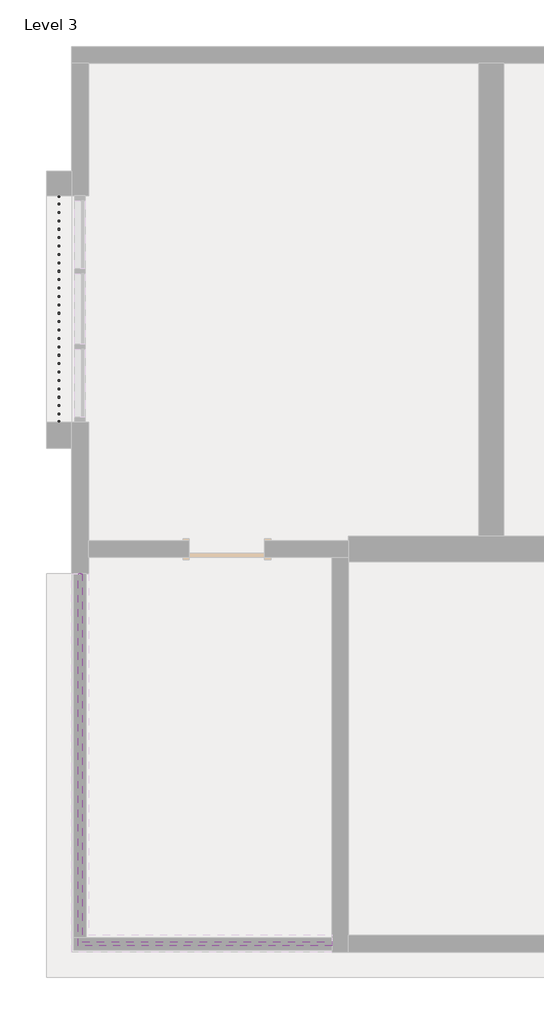
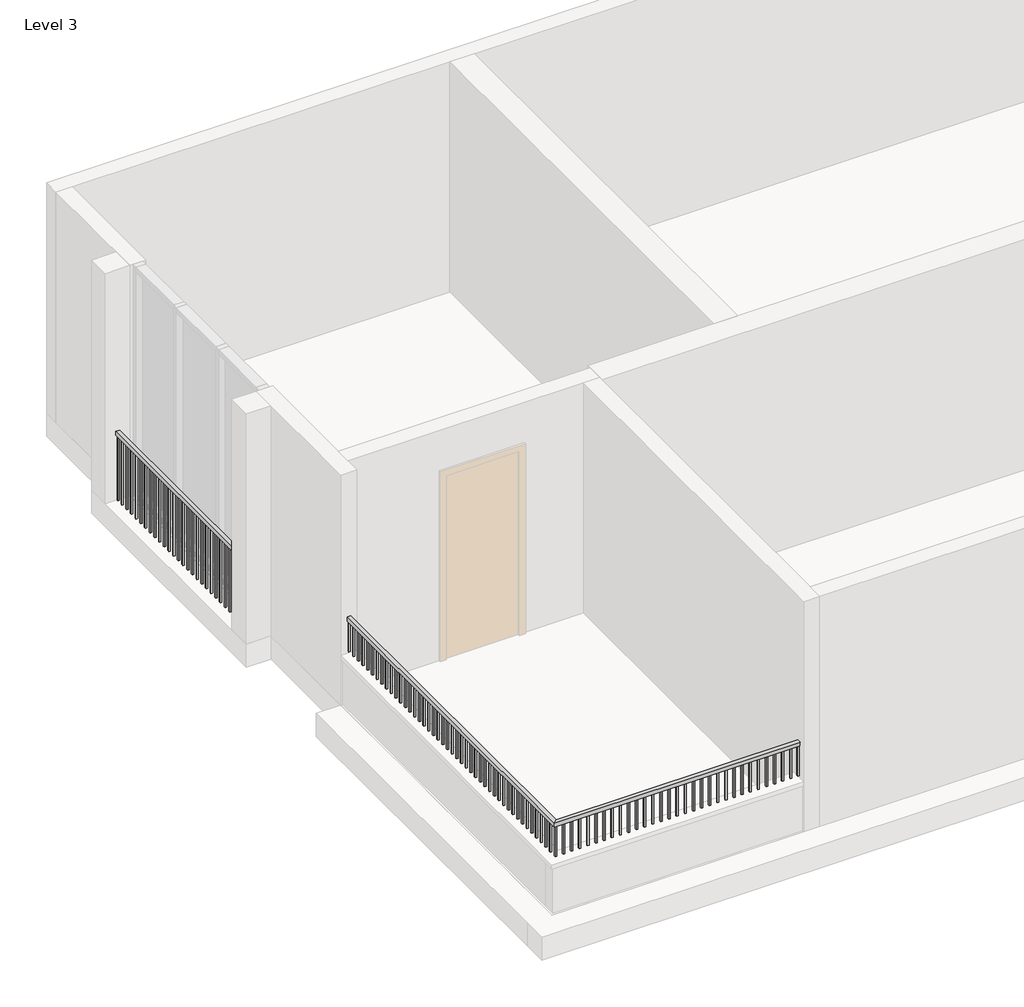
# One storey, part 2 of 2: 2 railings.
"""IFC4 building model written with IfcOpenShell, lengths in millimetres."""

from ifc_helpers import new_model, si_unit, frame, origin, place, context, project, spatial, polyline, outline, extrude, faceted_brep, element, save

model = new_model("IFC4")

# Units and contexts
model_context = context("Model", 3, world=origin())
ifc_project = project(units=[si_unit("LENGTHUNIT", "METRE", prefix="MILLI")], contexts=[model_context])

# Site, building, storey
site = spatial("IfcSite", under=ifc_project)
building = spatial("IfcBuilding", under=site)
storey = spatial("IfcBuildingStorey", under=building, Name="Level 3", Elevation=6096.0)

# Railings
placement = place(None, origin())
element("IfcRailing", 1, ObjectType="Handrail - Rectangular", at=placement, inside=storey, context=model_context, shape_type="SolidModel", body=[
    faceted_brep([(-15179.2169582, -9411.0617616, 7848.6), (-15179.2169582, -9411.0617616, 7797.8), (-15179.2169582, -9360.2617616, 7797.8), (-15179.2169582, -9360.2617616, 7848.6), (-18252.6169582, -9411.0617616, 7848.6), (-18252.6169582, -9411.0617616, 7797.8), (-18201.8169582, -9360.2617616, 7797.8), (-18201.8169582, -9360.2617616, 7848.6), (-18252.6169582, -4908.9117616, 7848.6), (-18201.8169582, -4908.9117616, 7848.6), (-18201.8169582, -4908.9117616, 7797.8), (-18252.6169582, -4908.9117616, 7797.8)], [[[0, 1, 2, 3]], [[1, 0, 4, 5]], [[2, 1, 5, 6]], [[3, 2, 6, 7]], [[0, 3, 7, 4]], [[8, 9, 10, 11]], [[5, 4, 8, 11]], [[6, 5, 11, 10]], [[7, 6, 10, 9]], [[4, 7, 9, 8]]]),
    extrude(outline(polyline([(-18217.6919582, -4924.7867616), (-18236.7419582, -4924.7867616), (-18236.7419582, -4905.7367616), (-18217.6919582, -4905.7367616), (-18217.6919582, -4924.7867616)])), frame((0.0, 0.0, 7391.4), z_axis=(0.0, 0.0, 1.0), x_axis=(1.0, 0.0, 0.0)), (0.0, 0.0, 1.0), 406.4),
    extrude(outline(polyline([(-18217.6919582, -5026.3867616), (-18236.7419582, -5026.3867616), (-18236.7419582, -5007.3367616), (-18217.6919582, -5007.3367616), (-18217.6919582, -5026.3867616)])), frame((0.0, 0.0, 7391.4), z_axis=(0.0, 0.0, 1.0), x_axis=(1.0, 0.0, 0.0)), (0.0, 0.0, 1.0), 406.4),
    extrude(outline(polyline([(-18217.6919582, -5127.9867616), (-18236.7419582, -5127.9867616), (-18236.7419582, -5108.9367616), (-18217.6919582, -5108.9367616), (-18217.6919582, -5127.9867616)])), frame((0.0, 0.0, 7391.4), z_axis=(0.0, 0.0, 1.0), x_axis=(1.0, 0.0, 0.0)), (0.0, 0.0, 1.0), 406.4),
    extrude(outline(polyline([(-18217.6919582, -5229.5867616), (-18236.7419582, -5229.5867616), (-18236.7419582, -5210.5367616), (-18217.6919582, -5210.5367616), (-18217.6919582, -5229.5867616)])), frame((0.0, 0.0, 7391.4), z_axis=(0.0, 0.0, 1.0), x_axis=(1.0, 0.0, 0.0)), (0.0, 0.0, 1.0), 406.4),
    extrude(outline(polyline([(-18217.6919582, -5331.1867616), (-18236.7419582, -5331.1867616), (-18236.7419582, -5312.1367616), (-18217.6919582, -5312.1367616), (-18217.6919582, -5331.1867616)])), frame((0.0, 0.0, 7391.4), z_axis=(0.0, 0.0, 1.0), x_axis=(1.0, 0.0, 0.0)), (0.0, 0.0, 1.0), 406.4),
    extrude(outline(polyline([(-18217.6919582, -5432.7867616), (-18236.7419582, -5432.7867616), (-18236.7419582, -5413.7367616), (-18217.6919582, -5413.7367616), (-18217.6919582, -5432.7867616)])), frame((0.0, 0.0, 7391.4), z_axis=(0.0, 0.0, 1.0), x_axis=(1.0, 0.0, 0.0)), (0.0, 0.0, 1.0), 406.4),
    extrude(outline(polyline([(-18217.6919582, -5534.3867616), (-18236.7419582, -5534.3867616), (-18236.7419582, -5515.3367616), (-18217.6919582, -5515.3367616), (-18217.6919582, -5534.3867616)])), frame((0.0, 0.0, 7391.4), z_axis=(0.0, 0.0, 1.0), x_axis=(1.0, 0.0, 0.0)), (0.0, 0.0, 1.0), 406.4),
    extrude(outline(polyline([(-18217.6919582, -5635.9867616), (-18236.7419582, -5635.9867616), (-18236.7419582, -5616.9367616), (-18217.6919582, -5616.9367616), (-18217.6919582, -5635.9867616)])), frame((0.0, 0.0, 7391.4), z_axis=(0.0, 0.0, 1.0), x_axis=(1.0, 0.0, 0.0)), (0.0, 0.0, 1.0), 406.4),
    extrude(outline(polyline([(-18217.6919582, -5737.5867616), (-18236.7419582, -5737.5867616), (-18236.7419582, -5718.5367616), (-18217.6919582, -5718.5367616), (-18217.6919582, -5737.5867616)])), frame((0.0, 0.0, 7391.4), z_axis=(0.0, 0.0, 1.0), x_axis=(1.0, 0.0, 0.0)), (0.0, 0.0, 1.0), 406.4),
    extrude(outline(polyline([(-18217.6919582, -5839.1867616), (-18236.7419582, -5839.1867616), (-18236.7419582, -5820.1367616), (-18217.6919582, -5820.1367616), (-18217.6919582, -5839.1867616)])), frame((0.0, 0.0, 7391.4), z_axis=(0.0, 0.0, 1.0), x_axis=(1.0, 0.0, 0.0)), (0.0, 0.0, 1.0), 406.4),
    extrude(outline(polyline([(-18217.6919582, -5940.7867616), (-18236.7419582, -5940.7867616), (-18236.7419582, -5921.7367616), (-18217.6919582, -5921.7367616), (-18217.6919582, -5940.7867616)])), frame((0.0, 0.0, 7391.4), z_axis=(0.0, 0.0, 1.0), x_axis=(1.0, 0.0, 0.0)), (0.0, 0.0, 1.0), 406.4),
    extrude(outline(polyline([(-18217.6919582, -6042.3867616), (-18236.7419582, -6042.3867616), (-18236.7419582, -6023.3367616), (-18217.6919582, -6023.3367616), (-18217.6919582, -6042.3867616)])), frame((0.0, 0.0, 7391.4), z_axis=(0.0, 0.0, 1.0), x_axis=(1.0, 0.0, 0.0)), (0.0, 0.0, 1.0), 406.4),
    extrude(outline(polyline([(-18217.6919582, -6143.9867616), (-18236.7419582, -6143.9867616), (-18236.7419582, -6124.9367616), (-18217.6919582, -6124.9367616), (-18217.6919582, -6143.9867616)])), frame((0.0, 0.0, 7391.4), z_axis=(0.0, 0.0, 1.0), x_axis=(1.0, 0.0, 0.0)), (0.0, 0.0, 1.0), 406.4),
    extrude(outline(polyline([(-18217.6919582, -6245.5867616), (-18236.7419582, -6245.5867616), (-18236.7419582, -6226.5367616), (-18217.6919582, -6226.5367616), (-18217.6919582, -6245.5867616)])), frame((0.0, 0.0, 7391.4), z_axis=(0.0, 0.0, 1.0), x_axis=(1.0, 0.0, 0.0)), (0.0, 0.0, 1.0), 406.4),
    extrude(outline(polyline([(-18217.6919582, -6347.1867616), (-18236.7419582, -6347.1867616), (-18236.7419582, -6328.1367616), (-18217.6919582, -6328.1367616), (-18217.6919582, -6347.1867616)])), frame((0.0, 0.0, 7391.4), z_axis=(0.0, 0.0, 1.0), x_axis=(1.0, 0.0, 0.0)), (0.0, 0.0, 1.0), 406.4),
    extrude(outline(polyline([(-18217.6919582, -6448.7867616), (-18236.7419582, -6448.7867616), (-18236.7419582, -6429.7367616), (-18217.6919582, -6429.7367616), (-18217.6919582, -6448.7867616)])), frame((0.0, 0.0, 7391.4), z_axis=(0.0, 0.0, 1.0), x_axis=(1.0, 0.0, 0.0)), (0.0, 0.0, 1.0), 406.4),
    extrude(outline(polyline([(-18217.6919582, -6550.3867616), (-18236.7419582, -6550.3867616), (-18236.7419582, -6531.3367616), (-18217.6919582, -6531.3367616), (-18217.6919582, -6550.3867616)])), frame((0.0, 0.0, 7391.4), z_axis=(0.0, 0.0, 1.0), x_axis=(1.0, 0.0, 0.0)), (0.0, 0.0, 1.0), 406.4),
    extrude(outline(polyline([(-18217.6919582, -6651.9867616), (-18236.7419582, -6651.9867616), (-18236.7419582, -6632.9367616), (-18217.6919582, -6632.9367616), (-18217.6919582, -6651.9867616)])), frame((0.0, 0.0, 7391.4), z_axis=(0.0, 0.0, 1.0), x_axis=(1.0, 0.0, 0.0)), (0.0, 0.0, 1.0), 406.4),
    extrude(outline(polyline([(-18217.6919582, -6753.5867616), (-18236.7419582, -6753.5867616), (-18236.7419582, -6734.5367616), (-18217.6919582, -6734.5367616), (-18217.6919582, -6753.5867616)])), frame((0.0, 0.0, 7391.4), z_axis=(0.0, 0.0, 1.0), x_axis=(1.0, 0.0, 0.0)), (0.0, 0.0, 1.0), 406.4),
    extrude(outline(polyline([(-18217.6919582, -6855.1867616), (-18236.7419582, -6855.1867616), (-18236.7419582, -6836.1367616), (-18217.6919582, -6836.1367616), (-18217.6919582, -6855.1867616)])), frame((0.0, 0.0, 7391.4), z_axis=(0.0, 0.0, 1.0), x_axis=(1.0, 0.0, 0.0)), (0.0, 0.0, 1.0), 406.4),
    extrude(outline(polyline([(-18217.6919582, -6956.7867616), (-18236.7419582, -6956.7867616), (-18236.7419582, -6937.7367616), (-18217.6919582, -6937.7367616), (-18217.6919582, -6956.7867616)])), frame((0.0, 0.0, 7391.4), z_axis=(0.0, 0.0, 1.0), x_axis=(1.0, 0.0, 0.0)), (0.0, 0.0, 1.0), 406.4),
    extrude(outline(polyline([(-18217.6919582, -7058.3867616), (-18236.7419582, -7058.3867616), (-18236.7419582, -7039.3367616), (-18217.6919582, -7039.3367616), (-18217.6919582, -7058.3867616)])), frame((0.0, 0.0, 7391.4), z_axis=(0.0, 0.0, 1.0), x_axis=(1.0, 0.0, 0.0)), (0.0, 0.0, 1.0), 406.4),
    extrude(outline(polyline([(-18217.6919582, -7159.9867616), (-18236.7419582, -7159.9867616), (-18236.7419582, -7140.9367616), (-18217.6919582, -7140.9367616), (-18217.6919582, -7159.9867616)])), frame((0.0, 0.0, 7391.4), z_axis=(0.0, 0.0, 1.0), x_axis=(1.0, 0.0, 0.0)), (0.0, 0.0, 1.0), 406.4),
    extrude(outline(polyline([(-18217.6919582, -7261.5867616), (-18236.7419582, -7261.5867616), (-18236.7419582, -7242.5367616), (-18217.6919582, -7242.5367616), (-18217.6919582, -7261.5867616)])), frame((0.0, 0.0, 7391.4), z_axis=(0.0, 0.0, 1.0), x_axis=(1.0, 0.0, 0.0)), (0.0, 0.0, 1.0), 406.4),
    extrude(outline(polyline([(-18217.6919582, -7363.1867616), (-18236.7419582, -7363.1867616), (-18236.7419582, -7344.1367616), (-18217.6919582, -7344.1367616), (-18217.6919582, -7363.1867616)])), frame((0.0, 0.0, 7391.4), z_axis=(0.0, 0.0, 1.0), x_axis=(1.0, 0.0, 0.0)), (0.0, 0.0, 1.0), 406.4),
    extrude(outline(polyline([(-18217.6919582, -7464.7867616), (-18236.7419582, -7464.7867616), (-18236.7419582, -7445.7367616), (-18217.6919582, -7445.7367616), (-18217.6919582, -7464.7867616)])), frame((0.0, 0.0, 7391.4), z_axis=(0.0, 0.0, 1.0), x_axis=(1.0, 0.0, 0.0)), (0.0, 0.0, 1.0), 406.4),
    extrude(outline(polyline([(-18217.6919582, -7566.3867616), (-18236.7419582, -7566.3867616), (-18236.7419582, -7547.3367616), (-18217.6919582, -7547.3367616), (-18217.6919582, -7566.3867616)])), frame((0.0, 0.0, 7391.4), z_axis=(0.0, 0.0, 1.0), x_axis=(1.0, 0.0, 0.0)), (0.0, 0.0, 1.0), 406.4),
    extrude(outline(polyline([(-18217.6919582, -7667.9867616), (-18236.7419582, -7667.9867616), (-18236.7419582, -7648.9367616), (-18217.6919582, -7648.9367616), (-18217.6919582, -7667.9867616)])), frame((0.0, 0.0, 7391.4), z_axis=(0.0, 0.0, 1.0), x_axis=(1.0, 0.0, 0.0)), (0.0, 0.0, 1.0), 406.4),
    extrude(outline(polyline([(-18217.6919582, -7769.5867616), (-18236.7419582, -7769.5867616), (-18236.7419582, -7750.5367616), (-18217.6919582, -7750.5367616), (-18217.6919582, -7769.5867616)])), frame((0.0, 0.0, 7391.4), z_axis=(0.0, 0.0, 1.0), x_axis=(1.0, 0.0, 0.0)), (0.0, 0.0, 1.0), 406.4),
    extrude(outline(polyline([(-18217.6919582, -7871.1867616), (-18236.7419582, -7871.1867616), (-18236.7419582, -7852.1367616), (-18217.6919582, -7852.1367616), (-18217.6919582, -7871.1867616)])), frame((0.0, 0.0, 7391.4), z_axis=(0.0, 0.0, 1.0), x_axis=(1.0, 0.0, 0.0)), (0.0, 0.0, 1.0), 406.4),
    extrude(outline(polyline([(-18217.6919582, -7972.7867616), (-18236.7419582, -7972.7867616), (-18236.7419582, -7953.7367616), (-18217.6919582, -7953.7367616), (-18217.6919582, -7972.7867616)])), frame((0.0, 0.0, 7391.4), z_axis=(0.0, 0.0, 1.0), x_axis=(1.0, 0.0, 0.0)), (0.0, 0.0, 1.0), 406.4),
    extrude(outline(polyline([(-18217.6919582, -8074.3867616), (-18236.7419582, -8074.3867616), (-18236.7419582, -8055.3367616), (-18217.6919582, -8055.3367616), (-18217.6919582, -8074.3867616)])), frame((0.0, 0.0, 7391.4), z_axis=(0.0, 0.0, 1.0), x_axis=(1.0, 0.0, 0.0)), (0.0, 0.0, 1.0), 406.4),
    extrude(outline(polyline([(-18217.6919582, -8175.9867616), (-18236.7419582, -8175.9867616), (-18236.7419582, -8156.9367616), (-18217.6919582, -8156.9367616), (-18217.6919582, -8175.9867616)])), frame((0.0, 0.0, 7391.4), z_axis=(0.0, 0.0, 1.0), x_axis=(1.0, 0.0, 0.0)), (0.0, 0.0, 1.0), 406.4),
    extrude(outline(polyline([(-18217.6919582, -8277.5867616), (-18236.7419582, -8277.5867616), (-18236.7419582, -8258.5367616), (-18217.6919582, -8258.5367616), (-18217.6919582, -8277.5867616)])), frame((0.0, 0.0, 7391.4), z_axis=(0.0, 0.0, 1.0), x_axis=(1.0, 0.0, 0.0)), (0.0, 0.0, 1.0), 406.4),
    extrude(outline(polyline([(-18217.6919582, -8379.1867616), (-18236.7419582, -8379.1867616), (-18236.7419582, -8360.1367616), (-18217.6919582, -8360.1367616), (-18217.6919582, -8379.1867616)])), frame((0.0, 0.0, 7391.4), z_axis=(0.0, 0.0, 1.0), x_axis=(1.0, 0.0, 0.0)), (0.0, 0.0, 1.0), 406.4),
    extrude(outline(polyline([(-18217.6919582, -8480.7867616), (-18236.7419582, -8480.7867616), (-18236.7419582, -8461.7367616), (-18217.6919582, -8461.7367616), (-18217.6919582, -8480.7867616)])), frame((0.0, 0.0, 7391.4), z_axis=(0.0, 0.0, 1.0), x_axis=(1.0, 0.0, 0.0)), (0.0, 0.0, 1.0), 406.4),
    extrude(outline(polyline([(-18217.6919582, -8582.3867616), (-18236.7419582, -8582.3867616), (-18236.7419582, -8563.3367616), (-18217.6919582, -8563.3367616), (-18217.6919582, -8582.3867616)])), frame((0.0, 0.0, 7391.4), z_axis=(0.0, 0.0, 1.0), x_axis=(1.0, 0.0, 0.0)), (0.0, 0.0, 1.0), 406.4),
    extrude(outline(polyline([(-18217.6919582, -8683.9867616), (-18236.7419582, -8683.9867616), (-18236.7419582, -8664.9367616), (-18217.6919582, -8664.9367616), (-18217.6919582, -8683.9867616)])), frame((0.0, 0.0, 7391.4), z_axis=(0.0, 0.0, 1.0), x_axis=(1.0, 0.0, 0.0)), (0.0, 0.0, 1.0), 406.4),
    extrude(outline(polyline([(-18217.6919582, -8785.5867616), (-18236.7419582, -8785.5867616), (-18236.7419582, -8766.5367616), (-18217.6919582, -8766.5367616), (-18217.6919582, -8785.5867616)])), frame((0.0, 0.0, 7391.4), z_axis=(0.0, 0.0, 1.0), x_axis=(1.0, 0.0, 0.0)), (0.0, 0.0, 1.0), 406.4),
    extrude(outline(polyline([(-18217.6919582, -8887.1867616), (-18236.7419582, -8887.1867616), (-18236.7419582, -8868.1367616), (-18217.6919582, -8868.1367616), (-18217.6919582, -8887.1867616)])), frame((0.0, 0.0, 7391.4), z_axis=(0.0, 0.0, 1.0), x_axis=(1.0, 0.0, 0.0)), (0.0, 0.0, 1.0), 406.4),
    extrude(outline(polyline([(-18217.6919582, -8988.7867616), (-18236.7419582, -8988.7867616), (-18236.7419582, -8969.7367616), (-18217.6919582, -8969.7367616), (-18217.6919582, -8988.7867616)])), frame((0.0, 0.0, 7391.4), z_axis=(0.0, 0.0, 1.0), x_axis=(1.0, 0.0, 0.0)), (0.0, 0.0, 1.0), 406.4),
    extrude(outline(polyline([(-18217.6919582, -9090.3867616), (-18236.7419582, -9090.3867616), (-18236.7419582, -9071.3367616), (-18217.6919582, -9071.3367616), (-18217.6919582, -9090.3867616)])), frame((0.0, 0.0, 7391.4), z_axis=(0.0, 0.0, 1.0), x_axis=(1.0, 0.0, 0.0)), (0.0, 0.0, 1.0), 406.4),
    extrude(outline(polyline([(-18217.6919582, -9191.9867616), (-18236.7419582, -9191.9867616), (-18236.7419582, -9172.9367616), (-18217.6919582, -9172.9367616), (-18217.6919582, -9191.9867616)])), frame((0.0, 0.0, 7391.4), z_axis=(0.0, 0.0, 1.0), x_axis=(1.0, 0.0, 0.0)), (0.0, 0.0, 1.0), 406.4),
    extrude(outline(polyline([(-18217.6919582, -9293.5867616), (-18236.7419582, -9293.5867616), (-18236.7419582, -9274.5367616), (-18217.6919582, -9274.5367616), (-18217.6919582, -9293.5867616)])), frame((0.0, 0.0, 7391.4), z_axis=(0.0, 0.0, 1.0), x_axis=(1.0, 0.0, 0.0)), (0.0, 0.0, 1.0), 406.4),
    extrude(outline(polyline([(-18116.0919582, -9376.1367616), (-18116.0919582, -9395.1867616), (-18135.1419582, -9395.1867616), (-18135.1419582, -9376.1367616), (-18116.0919582, -9376.1367616)])), frame((0.0, 0.0, 7391.4), z_axis=(0.0, 0.0, 1.0), x_axis=(1.0, 0.0, 0.0)), (0.0, 0.0, 1.0), 406.4),
    extrude(outline(polyline([(-18014.4919582, -9376.1367616), (-18014.4919582, -9395.1867616), (-18033.5419582, -9395.1867616), (-18033.5419582, -9376.1367616), (-18014.4919582, -9376.1367616)])), frame((0.0, 0.0, 7391.4), z_axis=(0.0, 0.0, 1.0), x_axis=(1.0, 0.0, 0.0)), (0.0, 0.0, 1.0), 406.4),
    extrude(outline(polyline([(-17912.8919582, -9376.1367616), (-17912.8919582, -9395.1867616), (-17931.9419582, -9395.1867616), (-17931.9419582, -9376.1367616), (-17912.8919582, -9376.1367616)])), frame((0.0, 0.0, 7391.4), z_axis=(0.0, 0.0, 1.0), x_axis=(1.0, 0.0, 0.0)), (0.0, 0.0, 1.0), 406.4),
    extrude(outline(polyline([(-17811.2919582, -9376.1367616), (-17811.2919582, -9395.1867616), (-17830.3419582, -9395.1867616), (-17830.3419582, -9376.1367616), (-17811.2919582, -9376.1367616)])), frame((0.0, 0.0, 7391.4), z_axis=(0.0, 0.0, 1.0), x_axis=(1.0, 0.0, 0.0)), (0.0, 0.0, 1.0), 406.4),
    extrude(outline(polyline([(-17709.6919582, -9376.1367616), (-17709.6919582, -9395.1867616), (-17728.7419582, -9395.1867616), (-17728.7419582, -9376.1367616), (-17709.6919582, -9376.1367616)])), frame((0.0, 0.0, 7391.4), z_axis=(0.0, 0.0, 1.0), x_axis=(1.0, 0.0, 0.0)), (0.0, 0.0, 1.0), 406.4),
    extrude(outline(polyline([(-17608.0919582, -9376.1367616), (-17608.0919582, -9395.1867616), (-17627.1419582, -9395.1867616), (-17627.1419582, -9376.1367616), (-17608.0919582, -9376.1367616)])), frame((0.0, 0.0, 7391.4), z_axis=(0.0, 0.0, 1.0), x_axis=(1.0, 0.0, 0.0)), (0.0, 0.0, 1.0), 406.4),
    extrude(outline(polyline([(-17506.4919582, -9376.1367616), (-17506.4919582, -9395.1867616), (-17525.5419582, -9395.1867616), (-17525.5419582, -9376.1367616), (-17506.4919582, -9376.1367616)])), frame((0.0, 0.0, 7391.4), z_axis=(0.0, 0.0, 1.0), x_axis=(1.0, 0.0, 0.0)), (0.0, 0.0, 1.0), 406.4),
    extrude(outline(polyline([(-17404.8919582, -9376.1367616), (-17404.8919582, -9395.1867616), (-17423.9419582, -9395.1867616), (-17423.9419582, -9376.1367616), (-17404.8919582, -9376.1367616)])), frame((0.0, 0.0, 7391.4), z_axis=(0.0, 0.0, 1.0), x_axis=(1.0, 0.0, 0.0)), (0.0, 0.0, 1.0), 406.4),
    extrude(outline(polyline([(-17303.2919582, -9376.1367616), (-17303.2919582, -9395.1867616), (-17322.3419582, -9395.1867616), (-17322.3419582, -9376.1367616), (-17303.2919582, -9376.1367616)])), frame((0.0, 0.0, 7391.4), z_axis=(0.0, 0.0, 1.0), x_axis=(1.0, 0.0, 0.0)), (0.0, 0.0, 1.0), 406.4),
    extrude(outline(polyline([(-17201.6919582, -9376.1367616), (-17201.6919582, -9395.1867616), (-17220.7419582, -9395.1867616), (-17220.7419582, -9376.1367616), (-17201.6919582, -9376.1367616)])), frame((0.0, 0.0, 7391.4), z_axis=(0.0, 0.0, 1.0), x_axis=(1.0, 0.0, 0.0)), (0.0, 0.0, 1.0), 406.4),
    extrude(outline(polyline([(-17100.0919582, -9376.1367616), (-17100.0919582, -9395.1867616), (-17119.1419582, -9395.1867616), (-17119.1419582, -9376.1367616), (-17100.0919582, -9376.1367616)])), frame((0.0, 0.0, 7391.4), z_axis=(0.0, 0.0, 1.0), x_axis=(1.0, 0.0, 0.0)), (0.0, 0.0, 1.0), 406.4),
    extrude(outline(polyline([(-16998.4919582, -9376.1367616), (-16998.4919582, -9395.1867616), (-17017.5419582, -9395.1867616), (-17017.5419582, -9376.1367616), (-16998.4919582, -9376.1367616)])), frame((0.0, 0.0, 7391.4), z_axis=(0.0, 0.0, 1.0), x_axis=(1.0, 0.0, 0.0)), (0.0, 0.0, 1.0), 406.4),
    extrude(outline(polyline([(-16896.8919582, -9376.1367616), (-16896.8919582, -9395.1867616), (-16915.9419582, -9395.1867616), (-16915.9419582, -9376.1367616), (-16896.8919582, -9376.1367616)])), frame((0.0, 0.0, 7391.4), z_axis=(0.0, 0.0, 1.0), x_axis=(1.0, 0.0, 0.0)), (0.0, 0.0, 1.0), 406.4),
    extrude(outline(polyline([(-16795.2919582, -9376.1367616), (-16795.2919582, -9395.1867616), (-16814.3419582, -9395.1867616), (-16814.3419582, -9376.1367616), (-16795.2919582, -9376.1367616)])), frame((0.0, 0.0, 7391.4), z_axis=(0.0, 0.0, 1.0), x_axis=(1.0, 0.0, 0.0)), (0.0, 0.0, 1.0), 406.4),
    extrude(outline(polyline([(-16693.6919582, -9376.1367616), (-16693.6919582, -9395.1867616), (-16712.7419582, -9395.1867616), (-16712.7419582, -9376.1367616), (-16693.6919582, -9376.1367616)])), frame((0.0, 0.0, 7391.4), z_axis=(0.0, 0.0, 1.0), x_axis=(1.0, 0.0, 0.0)), (0.0, 0.0, 1.0), 406.4),
    extrude(outline(polyline([(-16592.0919582, -9376.1367616), (-16592.0919582, -9395.1867616), (-16611.1419582, -9395.1867616), (-16611.1419582, -9376.1367616), (-16592.0919582, -9376.1367616)])), frame((0.0, 0.0, 7391.4), z_axis=(0.0, 0.0, 1.0), x_axis=(1.0, 0.0, 0.0)), (0.0, 0.0, 1.0), 406.4),
    extrude(outline(polyline([(-16490.4919582, -9376.1367616), (-16490.4919582, -9395.1867616), (-16509.5419582, -9395.1867616), (-16509.5419582, -9376.1367616), (-16490.4919582, -9376.1367616)])), frame((0.0, 0.0, 7391.4), z_axis=(0.0, 0.0, 1.0), x_axis=(1.0, 0.0, 0.0)), (0.0, 0.0, 1.0), 406.4),
    extrude(outline(polyline([(-16388.8919582, -9376.1367616), (-16388.8919582, -9395.1867616), (-16407.9419582, -9395.1867616), (-16407.9419582, -9376.1367616), (-16388.8919582, -9376.1367616)])), frame((0.0, 0.0, 7391.4), z_axis=(0.0, 0.0, 1.0), x_axis=(1.0, 0.0, 0.0)), (0.0, 0.0, 1.0), 406.4),
    extrude(outline(polyline([(-16287.2919582, -9376.1367616), (-16287.2919582, -9395.1867616), (-16306.3419582, -9395.1867616), (-16306.3419582, -9376.1367616), (-16287.2919582, -9376.1367616)])), frame((0.0, 0.0, 7391.4), z_axis=(0.0, 0.0, 1.0), x_axis=(1.0, 0.0, 0.0)), (0.0, 0.0, 1.0), 406.4),
    extrude(outline(polyline([(-16185.6919582, -9376.1367616), (-16185.6919582, -9395.1867616), (-16204.7419582, -9395.1867616), (-16204.7419582, -9376.1367616), (-16185.6919582, -9376.1367616)])), frame((0.0, 0.0, 7391.4), z_axis=(0.0, 0.0, 1.0), x_axis=(1.0, 0.0, 0.0)), (0.0, 0.0, 1.0), 406.4),
    extrude(outline(polyline([(-16084.0919582, -9376.1367616), (-16084.0919582, -9395.1867616), (-16103.1419582, -9395.1867616), (-16103.1419582, -9376.1367616), (-16084.0919582, -9376.1367616)])), frame((0.0, 0.0, 7391.4), z_axis=(0.0, 0.0, 1.0), x_axis=(1.0, 0.0, 0.0)), (0.0, 0.0, 1.0), 406.4),
    extrude(outline(polyline([(-15982.4919582, -9376.1367616), (-15982.4919582, -9395.1867616), (-16001.5419582, -9395.1867616), (-16001.5419582, -9376.1367616), (-15982.4919582, -9376.1367616)])), frame((0.0, 0.0, 7391.4), z_axis=(0.0, 0.0, 1.0), x_axis=(1.0, 0.0, 0.0)), (0.0, 0.0, 1.0), 406.4),
    extrude(outline(polyline([(-15880.8919582, -9376.1367616), (-15880.8919582, -9395.1867616), (-15899.9419582, -9395.1867616), (-15899.9419582, -9376.1367616), (-15880.8919582, -9376.1367616)])), frame((0.0, 0.0, 7391.4), z_axis=(0.0, 0.0, 1.0), x_axis=(1.0, 0.0, 0.0)), (0.0, 0.0, 1.0), 406.4),
    extrude(outline(polyline([(-15779.2919582, -9376.1367616), (-15779.2919582, -9395.1867616), (-15798.3419582, -9395.1867616), (-15798.3419582, -9376.1367616), (-15779.2919582, -9376.1367616)])), frame((0.0, 0.0, 7391.4), z_axis=(0.0, 0.0, 1.0), x_axis=(1.0, 0.0, 0.0)), (0.0, 0.0, 1.0), 406.4),
    extrude(outline(polyline([(-15677.6919582, -9376.1367616), (-15677.6919582, -9395.1867616), (-15696.7419582, -9395.1867616), (-15696.7419582, -9376.1367616), (-15677.6919582, -9376.1367616)])), frame((0.0, 0.0, 7391.4), z_axis=(0.0, 0.0, 1.0), x_axis=(1.0, 0.0, 0.0)), (0.0, 0.0, 1.0), 406.4),
    extrude(outline(polyline([(-15576.0919582, -9376.1367616), (-15576.0919582, -9395.1867616), (-15595.1419582, -9395.1867616), (-15595.1419582, -9376.1367616), (-15576.0919582, -9376.1367616)])), frame((0.0, 0.0, 7391.4), z_axis=(0.0, 0.0, 1.0), x_axis=(1.0, 0.0, 0.0)), (0.0, 0.0, 1.0), 406.4),
    extrude(outline(polyline([(-15474.4919582, -9376.1367616), (-15474.4919582, -9395.1867616), (-15493.5419582, -9395.1867616), (-15493.5419582, -9376.1367616), (-15474.4919582, -9376.1367616)])), frame((0.0, 0.0, 7391.4), z_axis=(0.0, 0.0, 1.0), x_axis=(1.0, 0.0, 0.0)), (0.0, 0.0, 1.0), 406.4),
    extrude(outline(polyline([(-15372.8919582, -9376.1367616), (-15372.8919582, -9395.1867616), (-15391.9419582, -9395.1867616), (-15391.9419582, -9376.1367616), (-15372.8919582, -9376.1367616)])), frame((0.0, 0.0, 7391.4), z_axis=(0.0, 0.0, 1.0), x_axis=(1.0, 0.0, 0.0)), (0.0, 0.0, 1.0), 406.4),
    extrude(outline(polyline([(-15271.2919582, -9376.1367616), (-15271.2919582, -9395.1867616), (-15290.3419582, -9395.1867616), (-15290.3419582, -9376.1367616), (-15271.2919582, -9376.1367616)])), frame((0.0, 0.0, 7391.4), z_axis=(0.0, 0.0, 1.0), x_axis=(1.0, 0.0, 0.0)), (0.0, 0.0, 1.0), 406.4),
    extrude(outline(polyline([(-18217.6919582, -9376.1367616), (-18217.6919582, -9395.1867616), (-18236.7419582, -9395.1867616), (-18236.7419582, -9376.1367616), (-18217.6919582, -9376.1367616)])), frame((0.0, 0.0, 7391.4), z_axis=(0.0, 0.0, 1.0), x_axis=(1.0, 0.0, 0.0)), (0.0, 0.0, 1.0), 406.4),
    extrude(outline(polyline([(-18217.6919582, -4927.9617616), (-18236.7419582, -4927.9617616), (-18236.7419582, -4908.9117616), (-18217.6919582, -4908.9117616), (-18217.6919582, -4927.9617616)])), frame((0.0, 0.0, 7391.4), z_axis=(0.0, 0.0, 1.0), x_axis=(1.0, 0.0, 0.0)), (0.0, 0.0, 1.0), 406.4),
    extrude(outline(polyline([(-15179.2169582, -9376.1367616), (-15179.2169582, -9395.1867616), (-15198.2669582, -9395.1867616), (-15198.2669582, -9376.1367616), (-15179.2169582, -9376.1367616)])), frame((0.0, 0.0, 7391.4), z_axis=(0.0, 0.0, 1.0), x_axis=(1.0, 0.0, 0.0)), (0.0, 0.0, 1.0), 406.4),
])
element("IfcRailing", 2, ObjectType="Handrail - Rectangular 2", at=placement, inside=storey, context=model_context, shape_type="SweptSolid", body=[
    extrude(outline(polyline([(-18506.6169582, -336.9117616), (-18455.8169582, -336.9117616), (-18455.8169582, -3080.1117616), (-18506.6169582, -3080.1117616), (-18506.6169582, -336.9117616)])), frame((0.0, 0.0, 7569.2), z_axis=(0.0, 0.0, 1.0), x_axis=(1.0, 0.0, 0.0)), (0.0, 0.0, 1.0), 50.8),
    extrude(outline(polyline([(-18490.7419582, -2968.9867616), (-18471.6919582, -2968.9867616), (-18471.6919582, -2988.0367616), (-18490.7419582, -2988.0367616), (-18490.7419582, -2968.9867616)])), frame((0.0, 0.0, 6705.6), z_axis=(0.0, 0.0, 1.0), x_axis=(1.0, 0.0, 0.0)), (0.0, 0.0, 1.0), 863.6),
    extrude(outline(polyline([(-18490.7419582, -2867.3867616), (-18471.6919582, -2867.3867616), (-18471.6919582, -2886.4367616), (-18490.7419582, -2886.4367616), (-18490.7419582, -2867.3867616)])), frame((0.0, 0.0, 6705.6), z_axis=(0.0, 0.0, 1.0), x_axis=(1.0, 0.0, 0.0)), (0.0, 0.0, 1.0), 863.6),
    extrude(outline(polyline([(-18490.7419582, -2765.7867616), (-18471.6919582, -2765.7867616), (-18471.6919582, -2784.8367616), (-18490.7419582, -2784.8367616), (-18490.7419582, -2765.7867616)])), frame((0.0, 0.0, 6705.6), z_axis=(0.0, 0.0, 1.0), x_axis=(1.0, 0.0, 0.0)), (0.0, 0.0, 1.0), 863.6),
    extrude(outline(polyline([(-18490.7419582, -2664.1867616), (-18471.6919582, -2664.1867616), (-18471.6919582, -2683.2367616), (-18490.7419582, -2683.2367616), (-18490.7419582, -2664.1867616)])), frame((0.0, 0.0, 6705.6), z_axis=(0.0, 0.0, 1.0), x_axis=(1.0, 0.0, 0.0)), (0.0, 0.0, 1.0), 863.6),
    extrude(outline(polyline([(-18490.7419582, -2562.5867616), (-18471.6919582, -2562.5867616), (-18471.6919582, -2581.6367616), (-18490.7419582, -2581.6367616), (-18490.7419582, -2562.5867616)])), frame((0.0, 0.0, 6705.6), z_axis=(0.0, 0.0, 1.0), x_axis=(1.0, 0.0, 0.0)), (0.0, 0.0, 1.0), 863.6),
    extrude(outline(polyline([(-18490.7419582, -2460.9867616), (-18471.6919582, -2460.9867616), (-18471.6919582, -2480.0367616), (-18490.7419582, -2480.0367616), (-18490.7419582, -2460.9867616)])), frame((0.0, 0.0, 6705.6), z_axis=(0.0, 0.0, 1.0), x_axis=(1.0, 0.0, 0.0)), (0.0, 0.0, 1.0), 863.6),
    extrude(outline(polyline([(-18490.7419582, -2359.3867616), (-18471.6919582, -2359.3867616), (-18471.6919582, -2378.4367616), (-18490.7419582, -2378.4367616), (-18490.7419582, -2359.3867616)])), frame((0.0, 0.0, 6705.6), z_axis=(0.0, 0.0, 1.0), x_axis=(1.0, 0.0, 0.0)), (0.0, 0.0, 1.0), 863.6),
    extrude(outline(polyline([(-18490.7419582, -2257.7867616), (-18471.6919582, -2257.7867616), (-18471.6919582, -2276.8367616), (-18490.7419582, -2276.8367616), (-18490.7419582, -2257.7867616)])), frame((0.0, 0.0, 6705.6), z_axis=(0.0, 0.0, 1.0), x_axis=(1.0, 0.0, 0.0)), (0.0, 0.0, 1.0), 863.6),
    extrude(outline(polyline([(-18490.7419582, -2156.1867616), (-18471.6919582, -2156.1867616), (-18471.6919582, -2175.2367616), (-18490.7419582, -2175.2367616), (-18490.7419582, -2156.1867616)])), frame((0.0, 0.0, 6705.6), z_axis=(0.0, 0.0, 1.0), x_axis=(1.0, 0.0, 0.0)), (0.0, 0.0, 1.0), 863.6),
    extrude(outline(polyline([(-18490.7419582, -2054.5867616), (-18471.6919582, -2054.5867616), (-18471.6919582, -2073.6367616), (-18490.7419582, -2073.6367616), (-18490.7419582, -2054.5867616)])), frame((0.0, 0.0, 6705.6), z_axis=(0.0, 0.0, 1.0), x_axis=(1.0, 0.0, 0.0)), (0.0, 0.0, 1.0), 863.6),
    extrude(outline(polyline([(-18490.7419582, -1952.9867616), (-18471.6919582, -1952.9867616), (-18471.6919582, -1972.0367616), (-18490.7419582, -1972.0367616), (-18490.7419582, -1952.9867616)])), frame((0.0, 0.0, 6705.6), z_axis=(0.0, 0.0, 1.0), x_axis=(1.0, 0.0, 0.0)), (0.0, 0.0, 1.0), 863.6),
    extrude(outline(polyline([(-18490.7419582, -1851.3867616), (-18471.6919582, -1851.3867616), (-18471.6919582, -1870.4367616), (-18490.7419582, -1870.4367616), (-18490.7419582, -1851.3867616)])), frame((0.0, 0.0, 6705.6), z_axis=(0.0, 0.0, 1.0), x_axis=(1.0, 0.0, 0.0)), (0.0, 0.0, 1.0), 863.6),
    extrude(outline(polyline([(-18490.7419582, -1749.7867616), (-18471.6919582, -1749.7867616), (-18471.6919582, -1768.8367616), (-18490.7419582, -1768.8367616), (-18490.7419582, -1749.7867616)])), frame((0.0, 0.0, 6705.6), z_axis=(0.0, 0.0, 1.0), x_axis=(1.0, 0.0, 0.0)), (0.0, 0.0, 1.0), 863.6),
    extrude(outline(polyline([(-18490.7419582, -1648.1867616), (-18471.6919582, -1648.1867616), (-18471.6919582, -1667.2367616), (-18490.7419582, -1667.2367616), (-18490.7419582, -1648.1867616)])), frame((0.0, 0.0, 6705.6), z_axis=(0.0, 0.0, 1.0), x_axis=(1.0, 0.0, 0.0)), (0.0, 0.0, 1.0), 863.6),
    extrude(outline(polyline([(-18490.7419582, -1546.5867616), (-18471.6919582, -1546.5867616), (-18471.6919582, -1565.6367616), (-18490.7419582, -1565.6367616), (-18490.7419582, -1546.5867616)])), frame((0.0, 0.0, 6705.6), z_axis=(0.0, 0.0, 1.0), x_axis=(1.0, 0.0, 0.0)), (0.0, 0.0, 1.0), 863.6),
    extrude(outline(polyline([(-18490.7419582, -1444.9867616), (-18471.6919582, -1444.9867616), (-18471.6919582, -1464.0367616), (-18490.7419582, -1464.0367616), (-18490.7419582, -1444.9867616)])), frame((0.0, 0.0, 6705.6), z_axis=(0.0, 0.0, 1.0), x_axis=(1.0, 0.0, 0.0)), (0.0, 0.0, 1.0), 863.6),
    extrude(outline(polyline([(-18490.7419582, -1343.3867616), (-18471.6919582, -1343.3867616), (-18471.6919582, -1362.4367616), (-18490.7419582, -1362.4367616), (-18490.7419582, -1343.3867616)])), frame((0.0, 0.0, 6705.6), z_axis=(0.0, 0.0, 1.0), x_axis=(1.0, 0.0, 0.0)), (0.0, 0.0, 1.0), 863.6),
    extrude(outline(polyline([(-18490.7419582, -1241.7867616), (-18471.6919582, -1241.7867616), (-18471.6919582, -1260.8367616), (-18490.7419582, -1260.8367616), (-18490.7419582, -1241.7867616)])), frame((0.0, 0.0, 6705.6), z_axis=(0.0, 0.0, 1.0), x_axis=(1.0, 0.0, 0.0)), (0.0, 0.0, 1.0), 863.6),
    extrude(outline(polyline([(-18490.7419582, -1140.1867616), (-18471.6919582, -1140.1867616), (-18471.6919582, -1159.2367616), (-18490.7419582, -1159.2367616), (-18490.7419582, -1140.1867616)])), frame((0.0, 0.0, 6705.6), z_axis=(0.0, 0.0, 1.0), x_axis=(1.0, 0.0, 0.0)), (0.0, 0.0, 1.0), 863.6),
    extrude(outline(polyline([(-18490.7419582, -1038.5867616), (-18471.6919582, -1038.5867616), (-18471.6919582, -1057.6367616), (-18490.7419582, -1057.6367616), (-18490.7419582, -1038.5867616)])), frame((0.0, 0.0, 6705.6), z_axis=(0.0, 0.0, 1.0), x_axis=(1.0, 0.0, 0.0)), (0.0, 0.0, 1.0), 863.6),
    extrude(outline(polyline([(-18490.7419582, -936.9867616), (-18471.6919582, -936.9867616), (-18471.6919582, -956.0367616), (-18490.7419582, -956.0367616), (-18490.7419582, -936.9867616)])), frame((0.0, 0.0, 6705.6), z_axis=(0.0, 0.0, 1.0), x_axis=(1.0, 0.0, 0.0)), (0.0, 0.0, 1.0), 863.6),
    extrude(outline(polyline([(-18490.7419582, -835.3867616), (-18471.6919582, -835.3867616), (-18471.6919582, -854.4367616), (-18490.7419582, -854.4367616), (-18490.7419582, -835.3867616)])), frame((0.0, 0.0, 6705.6), z_axis=(0.0, 0.0, 1.0), x_axis=(1.0, 0.0, 0.0)), (0.0, 0.0, 1.0), 863.6),
    extrude(outline(polyline([(-18490.7419582, -733.7867616), (-18471.6919582, -733.7867616), (-18471.6919582, -752.8367616), (-18490.7419582, -752.8367616), (-18490.7419582, -733.7867616)])), frame((0.0, 0.0, 6705.6), z_axis=(0.0, 0.0, 1.0), x_axis=(1.0, 0.0, 0.0)), (0.0, 0.0, 1.0), 863.6),
    extrude(outline(polyline([(-18490.7419582, -632.1867616), (-18471.6919582, -632.1867616), (-18471.6919582, -651.2367616), (-18490.7419582, -651.2367616), (-18490.7419582, -632.1867616)])), frame((0.0, 0.0, 6705.6), z_axis=(0.0, 0.0, 1.0), x_axis=(1.0, 0.0, 0.0)), (0.0, 0.0, 1.0), 863.6),
    extrude(outline(polyline([(-18490.7419582, -530.5867616), (-18471.6919582, -530.5867616), (-18471.6919582, -549.6367616), (-18490.7419582, -549.6367616), (-18490.7419582, -530.5867616)])), frame((0.0, 0.0, 6705.6), z_axis=(0.0, 0.0, 1.0), x_axis=(1.0, 0.0, 0.0)), (0.0, 0.0, 1.0), 863.6),
    extrude(outline(polyline([(-18490.7419582, -428.9867616), (-18471.6919582, -428.9867616), (-18471.6919582, -448.0367616), (-18490.7419582, -448.0367616), (-18490.7419582, -428.9867616)])), frame((0.0, 0.0, 6705.6), z_axis=(0.0, 0.0, 1.0), x_axis=(1.0, 0.0, 0.0)), (0.0, 0.0, 1.0), 863.6),
    extrude(outline(polyline([(-18490.7419582, -3061.0617616), (-18471.6919582, -3061.0617616), (-18471.6919582, -3080.1117616), (-18490.7419582, -3080.1117616), (-18490.7419582, -3061.0617616)])), frame((0.0, 0.0, 6705.6), z_axis=(0.0, 0.0, 1.0), x_axis=(1.0, 0.0, 0.0)), (0.0, 0.0, 1.0), 863.6),
    extrude(outline(polyline([(-18490.7419582, -336.9117616), (-18471.6919582, -336.9117616), (-18471.6919582, -355.9617616), (-18490.7419582, -355.9617616), (-18490.7419582, -336.9117616)])), frame((0.0, 0.0, 6705.6), z_axis=(0.0, 0.0, 1.0), x_axis=(1.0, 0.0, 0.0)), (0.0, 0.0, 1.0), 863.6),
])

save(model, "model.ifc")

# Revit data of these elements
# Type "Handrail - Rectangular"
#   Assembly Code = "C2010400"
#   built-in parameter 1008612 = 0.0416667 (stored number, unit not read)
#   built-in parameter 1008611 = 0.0416667 (stored number, unit not read)
#   built-in parameter 1008609 = 0.333333 (stored number, unit not read)
#   built-in parameter 1008604 = 0.166667 (stored number, unit not read)
#   built-in parameter 1008603 = 0.166667 (stored number, unit not read)
#   Railing Height = 1' - 6"
#   built-in parameter 1008630 = 2
#   built-in parameter 1008610 = 2
#   built-in parameter 1008618 = Baluster - Square : 3/4"
# Type "Handrail - Rectangular 2"
#   Assembly Code = "C2010400"
#   built-in parameter 1008612 = 0.0416667 (stored number, unit not read)
#   built-in parameter 1008611 = 0.0416667 (stored number, unit not read)
#   built-in parameter 1008609 = 0.333333 (stored number, unit not read)
#   built-in parameter 1008604 = 0.166667 (stored number, unit not read)
#   built-in parameter 1008603 = 0.166667 (stored number, unit not read)
#   Railing Height = 3' - 0"
#   built-in parameter 1008630 = 2
#   built-in parameter 1008610 = 2
#   built-in parameter 1008618 = Baluster - Square : 3/4"
# Element 1 (IfcRailing, "Handrail - Rectangular")
#   built-in parameter 1008621 = 4.25 (stored number, unit not read)
#   Phase Created = New Construction
# Element 2 (IfcRailing, "Handrail - Rectangular 2")
#   built-in parameter 1008621 = 2 (stored number, unit not read)
#   Phase Created = New Construction
